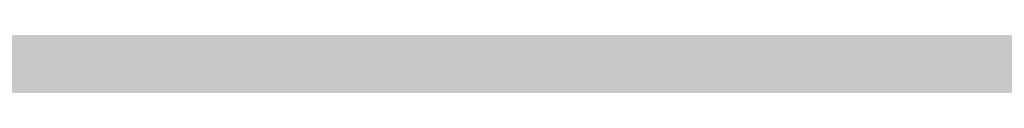
# Model space of a CAD drawing. Units: inches. Extents: x 2091 to 2899, y 967 to 2217.
# Tile 175 of 256: x 2203.151632 to 2203.161218, y 1152.24748 to 1152.2479. Entities that reach past the tile are written whole.
import ezdxf

# ---------------------------------------------------------------- set-up
doc = ezdxf.new("R2010")
doc.units = ezdxf.units.IN
doc.layers.add('A-WALL-PATT', color=141, linetype='Continuous', lineweight=13, true_color=0xadddf7)

msp = doc.modelspace()

# ---------------------------------------------------------------- hatches: boundary and pattern name
at = {"layer": 'A-WALL-PATT'}
h = msp.add_hatch(color=256, dxfattribs=at)
h.dxf.hatch_style = 1
h.paths.add_polyline_path([(2803.1436027, 2050.9190588), (2203.1436027, 2050.9190588), (2203.1436027, 1090.9190588), (2803.1436027, 1090.9190588)])
h.paths.add_polyline_path([(2635.7988501, 1147.5404649), (2674.5240524, 1147.5404649, 0.376086), (2678.5296653, 1152.8802017), (2678.5296653, 1159.5564734, 0.333335), (2674.524319, 1163.561846), (2674.524319, 1163.5618504), (2674.524319, 1192.9343904), (2635.8059707, 1192.9343904), (2597.0876225, 1192.9343904), (2597.0876225, 1163.561846, 0.333335), (2593.0822761, 1159.5564734), (2593.0822761, 1152.8802017, 0.376086), (2597.087889, 1147.5404649)], flags=0)
h.paths.add_polyline_path([(2436.0104329, 1278.2407784, 0.000483), (2435.9526433, 1278.215027, -0.001328), (2435.9356253, 1278.1116934, -0.001711), (2436.1164401, 1278.0407583, 0.002185)], flags=0)
h.paths.add_polyline_path([(2794.1436027, 1143.4190588), (2794.1436027, 1347.4190588), (2543.3701706, 1347.4190588), (2543.3701706, 1351.9190588), (2794.1436027, 1351.9190588), (2794.1436027, 1392.7135549), (2793.9473982, 1392.7135549), (2793.9473982, 1473.5368999), (2794.1436027, 1473.5368999), (2794.1436027, 1531.9190588), (2650.1436027, 1531.9190588), (2650.1436027, 1536.4190588), (2794.1436027, 1536.4190588), (2794.1436027, 1692.4190588), (2609.3756095, 1692.4190588), (2609.3756095, 1644.4190588), (2604.8756095, 1644.4190588), (2604.8756095, 1744.9190588), (2609.3756095, 1744.9190588), (2609.3756095, 1696.9190588), (2794.1436027, 1696.9190588), (2794.1436027, 1780.9190588), (2609.6436027, 1780.9190588), (2493.8756095, 1780.9190588), (2493.8756095, 1785.4190588), (2609.6436027, 1785.4190588), (2794.1436027, 1785.4190588), (2794.1436027, 1847.9388214), (2793.9512217, 1847.9388214), (2793.9512217, 1928.7621663), (2794.1436027, 1928.7621663), (2794.1436027, 1941.4190588), (2614.1436027, 1941.4190588), (2614.1436027, 1821.4190588), (2609.6436027, 1821.4190588), (2609.6436027, 1941.4190588), (2392.1436027, 1941.4190588), (2392.1436027, 1819.9190588), (2387.6436027, 1819.9190588), (2387.6436027, 1941.4190588), (2212.1436027, 1941.4190588), (2212.1436027, 1783.9190588), (2392.1436027, 1783.9190588), (2392.1436027, 1780.9190588), (2212.1436027, 1780.9190588), (2212.1436027, 1629.4190588), (2387.6436027, 1629.4190588), (2387.6436027, 1744.9190588), (2392.1436027, 1744.9190588), (2392.1436027, 1627.9190588), (2317.1436027, 1627.9190588), (2317.1436027, 1551.4190588), (2317.1436027, 1536.4190588), (2459.3835909, 1536.4190588), (2459.3835909, 1602.3964802), (2463.8835909, 1602.3964802), (2463.8835909, 1531.9190588), (2456.6436027, 1531.9190588), (2456.6436027, 1529.9190588), (2452.1436027, 1529.9190588), (2452.1436027, 1531.9190588), (2312.6436027, 1531.9190588), (2312.6436027, 1551.4190588), (2306.1436027, 1551.4190588), (2306.1436027, 1555.9190588), (2308.1436027, 1555.9190588), (2308.1436027, 1551.4190588), (2312.6436027, 1551.4190588), (2312.6436027, 1627.9190588), (2212.1436027, 1627.9190588), (2212.1436027, 1555.9190588), (2270.1436027, 1555.9190588), (2270.1436027, 1551.4190588), (2212.1436027, 1551.4190588), (2212.1436027, 1351.9190588), (2272.1436027, 1351.9190588), (2272.1436027, 1347.4190588), (2212.1436027, 1347.4190588), (2212.1436027, 1275.4190588), (2308.1436027, 1275.4190588), (2308.1436027, 1351.9190588), (2452.1436027, 1351.9190588), (2452.1436027, 1493.9190588), (2456.6436027, 1493.9190588), (2456.6436027, 1347.4190588), (2312.6436027, 1347.4190588), (2312.6436027, 1270.9190588), (2212.1436027, 1270.9190588), (2212.1436027, 1099.9190588), (2281.2375229, 1099.9190588), (2282.8710413, 1110.9138034), (2282.0083413, 1116.9966034), (2278.5577413, 1121.4204034), (2268.2056413, 1128.0562034), (2272.0876413, 1128.0562034), (2273.8129413, 1131.9270034), (2279.4203413, 1134.6919034), (2285.0278413, 1135.2449034), (2287.6158413, 1137.4568034), (2288.0471413, 1138.0098034), (2289.3411413, 1140.7747034), (2291.0665413, 1139.6687034), (2292.3605413, 1135.2449034), (2295.3798413, 1136.9038034), (2296.2425413, 1135.7979034), (2297.1052413, 1133.0330034), (2300.1246413, 1138.0098034), (2303.1439413, 1138.0098034), (2304.4379413, 1135.7979034), (2303.1439413, 1133.5860034), (2306.5946413, 1134.6919034), (2307.8887413, 1133.0330034), (2310.9080413, 1135.2449034), (2313.9274413, 1134.1389034), (2315.6268599, 1132.4271023), (2308.3200413, 1117.5496034), (2290.2038413, 1109.8079034), (2288.9098413, 1103.1721034), (2289.2723086, 1099.9190588), (2434.9182274, 1099.9190588), (2431.5932274, 1124.7880588), (2429.9302274, 1169.5530588), (2430.9271848, 1240.5196942), (2435.6589255, 1238.1861258), (2437.1352274, 1196.5540588), (2438.7982274, 1143.9730588), (2442.6782274, 1111.9980588), (2446.5582274, 1099.9190588), (2794.1436027, 1099.9190588), (2794.1436027, 1138.9190588), (2548.0324471, 1138.9190588), (2548.0324471, 1143.4190588), (2548.0324471, 1148.8190588), (2546.6684571, 1148.0315588), (2528.6856919, 1179.1786218, 0.256256), (2512.0324471, 1148.8190588), (2512.0324471, 1143.4190588), (2512.0324471, 1138.9190588), (2507.5324471, 1138.9190588), (2507.5324471, 1143.4190588), (2507.5324471, 1148.8190588, 0.256256), (2490.8792023, 1179.1786218), (2472.8964371, 1148.0315588), (2471.5324471, 1148.8190588), (2471.5324471, 1143.4190588), (2467.0324471, 1143.4190588), (2467.0324471, 1269.9457858, 0.039061), (2460.9099871, 1273.5800588), (2467.0324471, 1273.5800588), (2467.0324471, 1286.3253638, 0.014511), (2465.2161944, 1286.7619052), (2467.0324471, 1287.0525761), (2467.0324471, 1323.4190588), (2471.5324471, 1323.4190588), (2471.5324471, 1148.8190588), (2489.5324471, 1179.9959734), (2490.8964371, 1179.2084734), (2490.8792023, 1179.1786218, -0.256256), (2507.5324471, 1148.8190588), (2507.5324471, 1143.4190588), (2512.0324471, 1143.4190588), (2512.0324471, 1148.8190588, -0.256256), (2528.6856919, 1179.1786218), (2528.6684571, 1179.2084734), (2530.0324471, 1179.9959734), (2548.0324471, 1148.8190588), (2548.0324471, 1143.4190588)], flags=16)
h.paths.add_polyline_path([(2607.7685461, 1200.9450832), (2607.7685461, 1265.0306251), (2597.0876225, 1281.0520106), (2619.7845852, 1281.0520106), (2627.795278, 1337.1268598), (2635.7988501, 1337.1268598), (2643.8166634, 1337.1268598), (2651.8273562, 1281.0520106), (2674.524319, 1281.0520106), (2663.8433953, 1265.0306251), (2663.8433953, 1200.9450832), (2635.8059707, 1200.9450832)], flags=0)
edge = h.paths.add_edge_path(flags=0)
edge.add_ellipse((13303.8962153, 1272.9987247), major_axis=(-10595.3130399, 0.0000005), ratio=0.842303870086, start_angle=0.62823721906, end_angle=0.64655409989, ccw=False)
edge.add_ellipse((2711.7004495, 1156.8526781), major_axis=(2.2197691, 0), ratio=0.84230387, start_angle=111.5352435, end_angle=180.6282372, ccw=False)
edge.add_ellipse((13303.1562922, 1272.9987246), major_axis=(-10593.0263064, 0), ratio=0.842303869544, start_angle=0.52827147182, end_angle=0.64655409706, ccw=False)
edge.add_line((2710.7645961, 1175.3332951), (2710.1299858, 1175.3332951))
edge.add_ellipse((2710.1299858, 1176.5797752), major_axis=(1.4798461, 0), ratio=0.84230387, start_angle=180, end_angle=270, ccw=False)
edge.add_line((2708.6501397, 1176.5797752), (2708.6501397, 1200.7829144))
edge.add_ellipse((2710.1299858, 1200.7829144), major_axis=(1.4798461, 0), ratio=0.84230387, start_angle=90, end_angle=180, ccw=False)
edge.add_line((2710.1299858, 1202.0293944), (2710.4650752, 1202.0293944))
edge.add_ellipse((13303.1562922, 1272.9987246), major_axis=(-10593.0263064, 0), ratio=0.842303869544, start_angle=-0.09022908859, end_angle=0.38386677879, ccw=False)
edge.add_ellipse((2710.1299858, 1290.9270308), major_axis=(-1.4798461, 0), ratio=0.84230387, start_angle=0, end_angle=90, ccw=False)
edge.add_line((2708.6501397, 1290.9270308), (2708.6501397, 1315.13017))
edge.add_ellipse((2710.1299858, 1315.13017), major_axis=(-1.4798461, 0), ratio=0.84230387, start_angle=-90, end_angle=0, ccw=False)
edge.add_line((2710.1299858, 1316.3766501), (2710.7063141, 1316.3766501))
edge.add_ellipse((3238.4017202, 1296.2895655), major_axis=(528.2339998, 0), ratio=0.84230386954, start_angle=176.349572414, end_angle=177.820049686, ccw=False)
edge.add_ellipse((2775.0630432, 1071.4506962), major_axis=(313.3077613, 0), ratio=0.84230386954, start_angle=102.125965552, end_angle=103.780528989, ccw=False)
edge.add_ellipse((2775.0630432, 1078.3056979), major_axis=(-305.3028915, 0), ratio=0.84230386955, start_angle=-79.790461003, end_angle=-77.555372706, ccw=False)
edge.add_ellipse((2695.1417666, 1541.9753825), major_axis=(-250.9602162, 0), ratio=0.84230386954, start_angle=99.256566007, end_angle=102.554932644)
edge.add_line((2741.4103262, 1334.2142554), (2747.1325454, 1337.3784768))
edge.add_ellipse((2747.5386163, 1336.8574776), major_axis=(-0.739923, 0), ratio=0.84230387, start_angle=270, end_angle=307.9331305, ccw=False)
edge.add_ellipse((2747.5386163, 1336.8574776), major_axis=(-0.739923, 0), ratio=0.84230387, start_angle=232.0668695, end_angle=270, ccw=False)
edge.add_line((2747.9446872, 1337.3784768), (2753.6669064, 1334.2142554))
edge.add_ellipse((2799.935466, 1541.9753825), major_axis=(250.9602162, 0), ratio=0.84230386954, start_angle=257.445067356, end_angle=260.743433993)
edge.add_ellipse((2720.0141894, 1078.3056979), major_axis=(305.3028915, 0), ratio=0.84230386954, start_angle=77.555372707, end_angle=79.790461003, ccw=False)
edge.add_ellipse((2720.0141894, 1071.4506962), major_axis=(-313.3077613, 0), ratio=0.84230386954, start_angle=256.219471011, end_angle=257.874034448, ccw=False)
edge.add_ellipse((2256.6755124, 1296.2895655), major_axis=(-528.2339998, 0), ratio=0.84230386954, start_angle=182.179950314, end_angle=183.650427586, ccw=False)
edge.add_line((2784.3709184, 1316.3766501), (2784.9472468, 1316.3766501))
edge.add_ellipse((2784.9472468, 1315.13017), major_axis=(1.4798461, 0), ratio=0.84230387, start_angle=0, end_angle=90, ccw=False)
edge.add_line((2786.4270928, 1315.13017), (2786.4270928, 1290.9270308))
edge.add_ellipse((2784.9472468, 1290.9270308), major_axis=(1.4798461, 0), ratio=0.84230387, start_angle=270, end_angle=360, ccw=False)
edge.add_ellipse((-7808.0790596, 1272.9987246), major_axis=(10593.0263063, 0), ratio=0.842303869544, start_angle=-0.38386677879, end_angle=0.09022908859, ccw=False)
edge.add_line((2784.6121574, 1202.0293944), (2784.9472468, 1202.0293944))
edge.add_ellipse((2784.9472468, 1200.7829144), major_axis=(1.4798461, 0), ratio=0.84230387, start_angle=0, end_angle=90, ccw=False)
edge.add_line((2786.4270928, 1200.7829144), (2786.4270928, 1176.5797752))
edge.add_ellipse((2784.9472468, 1176.5797752), major_axis=(-1.4798461, 0), ratio=0.84230387, start_angle=90, end_angle=180, ccw=False)
edge.add_line((2784.9472468, 1175.3332951), (2784.3126365, 1175.3332951))
edge.add_ellipse((-7808.0790596, 1272.9987246), major_axis=(10593.0263063, 0), ratio=0.842303869544, start_angle=-0.61864319632, end_angle=-0.52827147182, ccw=False)
edge.add_ellipse((2783.3767831, 1156.8526781), major_axis=(-2.2197691, 0), ratio=0.84230387, start_angle=179.3717628, end_angle=248.4647566, ccw=False)
edge.add_ellipse((-7808.8189826, 1272.9987246), major_axis=(-10595.3130398, 0.0000036), ratio=0.842303865762, start_angle=179.3534459226, end_angle=179.37176280343, ccw=False)
edge.add_ellipse((2780.2973026, 1153.500793), major_axis=(-5.2464256, 0), ratio=0.84230387, start_angle=90, end_angle=179.3534459, ccw=False)
edge.add_line((2780.2973026, 1149.0817084), (2714.77993, 1149.0817084))
edge.add_ellipse((2714.77993, 1153.500793), major_axis=(5.2464256, 0), ratio=0.84230387, start_angle=180.6465541, end_angle=270, ccw=False)
edge = h.paths.add_edge_path(flags=0)
edge.add_line((2718.1873674, 1151.0078329), (2718.1873674, 1170.4723638))
edge.add_ellipse((2721.1470595, 1170.4723638), major_axis=(-2.9596921, 0), ratio=0.84230387, start_angle=-90, end_angle=0, ccw=False)
edge.add_line((2721.1470595, 1172.965324), (2773.9301731, 1172.965324))
edge.add_ellipse((2773.9301731, 1170.4723638), major_axis=(-2.9596921, 0), ratio=0.84230387, start_angle=180, end_angle=270, ccw=False)
edge.add_line((2776.8898652, 1170.4723638), (2776.8898652, 1151.0078329))
edge.add_line((2776.8898652, 1151.0078329), (2718.1873674, 1151.0078329))
edge = h.paths.add_edge_path(flags=0)
edge.add_line((2718.1873674, 1180.2341502), (2718.1873674, 1199.0578342))
edge.add_ellipse((2747.5386163, 1320.3986402), major_axis=(147.0179239, 0), ratio=0.84230386954, start_angle=256.40186531, end_angle=283.59813469)
edge.add_line((2776.8898652, 1199.0578342), (2776.8898652, 1180.2341502))
edge.add_ellipse((2747.5386163, 1301.5749562), major_axis=(147.0179239, 0), ratio=0.84230386954, start_angle=256.40186531, end_angle=283.59813469, ccw=False)
edge = h.paths.add_edge_path(flags=0)
edge.add_ellipse((13303.1562922, 1272.9987246), major_axis=(-10591.5464603, 0), ratio=0.842303869555, start_angle=0.05559431352, end_angle=0.37776419393, ccw=False)
edge.add_line((2711.6168595, 1262.7217103), (2715.6674076, 1249.4953957))
edge.add_ellipse((6413.8919626, 1241.691919), major_axis=(-3698.2361592, 0), ratio=0.842303869547, start_angle=-0.120897369, end_angle=0.3640763489)
edge.add_line((2715.7610383, 1218.1924547), (2711.9343065, 1203.167361))
edge = h.paths.add_edge_path(flags=0)
edge.add_line((2718.1873674, 1251.074566), (2716.0024854, 1267.4504351))
edge.add_ellipse((2742.1511746, 1202.1895399), major_axis=(81.7725845, 0), ratio=0.8423038695, start_angle=94.277420963, end_angle=111.834953797, ccw=False)
edge.add_line((2737.0097482, 1270.9306255), (2758.0674844, 1270.9306255))
edge.add_ellipse((2752.926058, 1202.1895399), major_axis=(81.7725845, 0), ratio=0.8423038695, start_angle=68.165046203, end_angle=85.722579037, ccw=False)
edge.add_line((2779.0747472, 1267.4504351), (2776.8898652, 1251.074566))
edge.add_ellipse((2750.3380588, 1187.8853558), major_axis=(79.5796641, 0), ratio=0.8423038695, start_angle=67.208085122, end_angle=85.129930403)
edge.add_line((2756.0346562, 1254.7436557), (2739.0425764, 1254.7436557))
edge.add_ellipse((2744.7391738, 1187.8853558), major_axis=(79.5796641, 0), ratio=0.8423038695, start_angle=94.870069597, end_angle=112.791914878)
edge = h.paths.add_edge_path(flags=0)
edge.add_line((2783.1429261, 1203.167361), (2779.3161943, 1218.1924547))
edge.add_ellipse((-918.81473, 1241.691919), major_axis=(3698.2361592, 0), ratio=0.842303869546, start_angle=-0.3640763489, end_angle=0.120897369)
edge.add_line((2779.409825, 1249.4953957), (2783.4603731, 1262.7217103))
edge.add_ellipse((-7808.0790596, 1272.9987246), major_axis=(-10591.5464603, 0), ratio=0.84230386954, start_angle=179.6222358061, end_angle=179.94440568651, ccw=False)
edge = h.paths.add_edge_path(flags=0)
edge.add_ellipse((2734.2008921, 1286.6904402), major_axis=(-0.3566086, 6.3400775), ratio=0.603833576, start_angle=89.00201428, end_angle=253.65740805, ccw=False)
edge.add_line((2730.3690013, 1286.5418057), (2730.3690013, 1301.3519803))
edge.add_line((2730.3690013, 1301.3519803), (2735.9133107, 1305.2148028))
edge.add_ellipse((2736.3849168, 1304.7345612), major_axis=(0.739923, 0), ratio=0.84230387, start_angle=90, end_angle=134.4802109, ccw=False)
edge.add_line((2736.3849168, 1305.3578013), (2738.0327829, 1305.3578013))
edge.add_line((2738.0327829, 1305.3578013), (2738.0327829, 1307.7079274))
edge.add_ellipse((2794.201642, 1307.7079274), major_axis=(56.168859, 0), ratio=0.8423038695, start_angle=150.5614304, end_angle=180, ccw=False)
edge.add_ellipse((2700.8755906, 1307.7079274), major_axis=(-56.168859, 0), ratio=0.8423038695, start_angle=180, end_angle=209.4385696, ccw=False)
edge.add_line((2757.0444497, 1307.7079274), (2757.0444497, 1305.3578013))
edge.add_line((2757.0444497, 1305.3578013), (2758.6923157, 1305.3578013))
edge.add_ellipse((2758.6923157, 1304.7345612), major_axis=(-0.739923, 0), ratio=0.84230387, start_angle=225.5197891, end_angle=270, ccw=False)
edge.add_line((2759.1639219, 1305.2148028), (2764.7082312, 1301.3519803))
edge.add_line((2764.7082312, 1301.3519803), (2764.7082312, 1286.5418057))
edge.add_ellipse((2760.8763405, 1286.6904402), major_axis=(0.3566086, 6.3400775), ratio=0.603833576, start_angle=106.34259195, end_angle=270.99798572, ccw=False)
edge.add_line((2757.0444497, 1285.7970896), (2757.0444497, 1307.7079274))
edge.add_ellipse((2700.8755906, 1307.7079274), major_axis=(-56.168859, 0), ratio=0.8423038695, start_angle=180, end_angle=209.4385696)
edge.add_ellipse((2794.201642, 1307.7079274), major_axis=(56.168859, 0), ratio=0.8423038695, start_angle=150.5614304, end_angle=180)
edge.add_line((2738.0327829, 1307.7079274), (2738.0327829, 1285.7970896))
h.paths.add_polyline_path([(2417.8122727, 1104.449704), (2413.4922727, 1102.529704), (2410.6122727, 1103.969704), (2409.1722727, 1106.369704), (2407.2522727, 1107.329704), (2406.2922727, 1109.729704), (2405.3322727, 1114.049704), (2405.3322727, 1117.889704), (2406.2922727, 1120.129704), (2407.2522727, 1119.809704), (2408.8483218, 1118.3276585), (2410.1739451, 1119.4241703), (2410.2112727, 1120.405704), (2411.0407305, 1121.4190541), (2410.6992727, 1119.858704), (2410.1739451, 1119.4241703), (2410.0884515, 1117.1761095), (2411.1328361, 1116.2063237), (2413.9722727, 1119.329704), (2416.8522727, 1120.769704), (2416.8697209, 1120.7987842), (2417.0350713, 1119.4051162), (2417.8962134, 1118.1433844), (2418.2922727, 1118.369704), (2419.5444467, 1120.0392692), (2419.3609153, 1118.387487), (2419.0321078, 1119.3561507), (2418.3989394, 1118.5119262), (2419.2522727, 1114.529704), (2418.7940909, 1107.1987949)], flags=0)
h.paths.add_polyline_path([(2508.8701706, 1347.4190588), (2508.3701706, 1347.4190588), (2508.3701706, 1351.9190588), (2508.8701706, 1351.9190588)], flags=0)
h.paths.add_polyline_path([(2473.3701706, 1347.4190588), (2472.3701706, 1347.4190588), (2467.8701706, 1347.4190588), (2467.8701706, 1455.4190588), (2472.3701706, 1455.4190588), (2472.3701706, 1352.4190588), (2473.3701706, 1352.4190588)], flags=0)
h.paths.add_polyline_path([(2352.106244, 1217.4461971), (2349.226244, 1218.8861971), (2347.786244, 1221.2861971), (2345.866244, 1222.2461971), (2344.906244, 1224.6461971), (2343.946244, 1228.9661971), (2343.946244, 1232.8061971), (2344.906244, 1235.0461971), (2345.866244, 1234.7261971), (2347.4622931, 1233.2441515), (2348.7879164, 1234.3406634), (2348.825244, 1235.3221971), (2349.6547018, 1236.3355471), (2349.313244, 1234.7751971), (2348.7879164, 1234.3406634), (2348.7024228, 1232.0926025), (2349.7468074, 1231.1228168), (2352.586244, 1234.2461971), (2355.466244, 1235.6861971), (2355.4836921, 1235.7152773), (2355.6490426, 1234.3216093), (2356.5101846, 1233.0598774), (2356.906244, 1233.2861971), (2358.1584179, 1234.9557623), (2357.9748866, 1233.3039801), (2357.6460791, 1234.2726438), (2357.0129107, 1233.4284193), (2357.866244, 1229.4461971), (2357.4080622, 1222.115288), (2356.426244, 1219.3661971)], flags=0)
h.paths.add_polyline_path([(2348.2967999, 1112.2244204), (2347.0137999, 1112.3104204), (2345.5297999, 1114.1274204), (2345.7317999, 1115.8584204), (2346.8117999, 1116.9824204), (2346.8117999, 1114.6464204), (2345.8667999, 1114.2144204), (2346.8797999, 1114.3004204)], flags=0)
h.paths.add_polyline_path([(2347.0137999, 1110.9264204), (2346.2717999, 1110.4934204), (2346.6097999, 1111.1864204)], flags=0)
h.paths.add_polyline_path([(2345.8667999, 1118.1944204), (2345.5297999, 1117.3294204), (2343.7077999, 1118.0214204), (2344.3827999, 1118.6264204)], flags=0)
h.paths.add_polyline_path([(2346.6767999, 1109.2824204), (2346.0697999, 1108.0714204), (2345.8667999, 1110.0614204)], flags=0)
h.paths.add_polyline_path([(2345.0567999, 1119.7514204), (2343.6397999, 1119.7514204), (2343.9777999, 1121.1354204)], flags=0)
h.paths.add_polyline_path([(2345.2597999, 1116.5504204), (2345.1247999, 1115.8584204), (2344.9217999, 1115.6854204), (2344.7197999, 1116.3774204)], flags=0)
h.paths.add_polyline_path([(2345.6647999, 1112.3104204), (2345.4617999, 1111.5324204), (2344.0447999, 1111.9644204), (2344.6517999, 1112.5704204)], flags=0)
h.paths.add_polyline_path([(2345.1917999, 1113.3494204), (2344.4497999, 1113.8684204), (2344.7197999, 1114.3874204)], flags=0)
h.paths.add_polyline_path([(2344.6517999, 1116.8094204), (2344.1797999, 1115.6854204), (2344.6517999, 1115.3394204), (2343.9097999, 1114.9064204), (2343.0327999, 1115.9444204), (2343.6397999, 1116.4634204)], flags=0)
h.paths.add_polyline_path([(2345.8667999, 1106.6864204), (2344.9897999, 1105.5624204), (2344.5167999, 1106.6004204)], flags=0)
h.paths.add_polyline_path([(2344.8547999, 1110.0614204), (2344.5167999, 1109.2824204), (2344.1127999, 1109.7154204)], flags=0)
h.paths.add_polyline_path([(2344.0447999, 1113.5224204), (2343.4377999, 1113.0894204), (2342.7627999, 1113.9544204)], flags=0)
h.paths.add_polyline_path([(2344.3147999, 1111.0124204), (2342.9647999, 1110.3204204), (2342.9647999, 1111.0994204)], flags=0)
h.paths.add_polyline_path([(2345.1247999, 1104.6974204), (2344.5847999, 1103.7454204), (2344.4497999, 1104.2644204)], flags=0)
h.paths.add_polyline_path([(2342.8297999, 1121.2224204), (2341.7497999, 1120.5304204), (2340.5357999, 1121.0494204), (2340.1307999, 1121.8284204), (2340.6707999, 1122.9524204), (2341.1427999, 1121.8284204), (2341.6147999, 1122.0014204)], flags=0)
h.paths.add_polyline_path([(2342.9647999, 1119.7514204), (2343.0327999, 1118.4534204), (2342.0877999, 1118.0214204), (2342.0197999, 1119.4914204)], flags=0)
h.paths.add_polyline_path([(2342.6947999, 1116.8964204), (2341.9527999, 1116.6364204), (2342.0197999, 1117.3294204)], flags=0)
h.paths.add_polyline_path([(2343.0327999, 1112.2244204), (2342.0197999, 1111.7914204), (2341.5477999, 1112.2244204), (2342.3577999, 1113.3494204)], flags=0)
h.paths.add_polyline_path([(2343.7747999, 1104.4374204), (2342.6277999, 1102.8804204), (2342.6947999, 1104.6104204), (2343.4377999, 1105.1294204)], flags=0)
h.paths.add_polyline_path([(2342.0197999, 1115.0794204), (2340.8057999, 1115.5124204), (2340.9407999, 1116.3774204)], flags=0)
h.paths.add_polyline_path([(2341.4807999, 1120.0974204), (2341.4807999, 1119.4054204), (2341.0757999, 1119.5784204), (2341.1427999, 1120.0974204)], flags=0)
h.paths.add_polyline_path([(2341.8177999, 1114.4734204), (2340.9407999, 1113.0894204), (2340.8057999, 1114.5604204)], flags=0)
h.paths.add_polyline_path([(2341.1427999, 1118.5404204), (2340.9407999, 1116.9824204), (2339.0507999, 1117.6754204), (2339.0507999, 1118.6264204)], flags=0)
h.paths.add_polyline_path([(2342.6947999, 1101.6684204), (2341.9527999, 1101.8414204), (2342.5597999, 1102.3614204)], flags=0)
h.paths.add_polyline_path([(2340.3327999, 1119.6654204), (2338.4437999, 1119.5784204), (2337.9037999, 1120.3574204), (2339.6577999, 1120.6164204)], flags=0)
h.paths.add_polyline_path([(2340.3327999, 1115.3394204), (2340.0627999, 1113.6954204), (2339.3877999, 1115.3394204)], flags=0)
h.paths.add_polyline_path([(2341.8177999, 1103.8314204), (2341.5477999, 1102.8804204), (2341.1427999, 1103.6584204)], flags=0)
h.paths.add_polyline_path([(2339.0507999, 1122.8664204), (2337.2957999, 1121.8284204), (2337.0937999, 1123.1254204), (2337.7687999, 1123.8184204)], flags=0)
h.paths.add_polyline_path([(2339.1177999, 1121.7414204), (2338.8477999, 1121.2224204), (2338.1737999, 1121.0494204), (2338.3757999, 1121.5684204)], flags=0)
h.paths.add_polyline_path([(2339.1857999, 1119.3194204), (2338.6457999, 1118.7134204), (2338.2407999, 1118.1074204), (2338.2407999, 1118.8864204)], flags=0)
h.paths.add_polyline_path([(2341.1427999, 1101.9284204), (2340.6027999, 1101.2364204), (2340.0627999, 1101.8414204), (2340.6027999, 1102.3614204)], flags=0)
h.paths.add_polyline_path([(2337.6337999, 1117.7614204), (2336.6207999, 1118.2804204), (2337.2957999, 1118.9724204)], flags=0)
h.paths.add_polyline_path([(2336.8237999, 1119.5784204), (2334.7987999, 1118.9724204), (2335.2037999, 1120.3574204), (2336.5537999, 1120.8764204)], flags=0)
h.paths.add_polyline_path([(2339.1177999, 1100.4574204), (2337.3637999, 1100.5434204), (2336.7557999, 1101.2364204)], flags=0)
h.paths.add_polyline_path([(2336.3507999, 1122.4334204), (2336.0137999, 1121.9144204), (2334.9337999, 1122.4334204), (2334.5287999, 1123.4714204), (2335.7437999, 1122.7794204)], flags=0)
h.paths.add_polyline_path([(2334.7317999, 1120.8764204), (2334.2587999, 1120.3574204), (2334.0567999, 1120.7894204), (2334.5967999, 1121.3084204)], flags=0)
h.paths.add_polyline_path([(2334.4617999, 1122.1744204), (2332.5717999, 1121.3084204), (2331.3567999, 1122.1744204), (2332.0997999, 1122.8664204)], flags=0)
h.paths.add_polyline_path([(2334.2587999, 1118.5404204), (2333.3817999, 1118.4534204), (2333.6517999, 1119.3194204)], flags=0)
h.paths.add_polyline_path([(2335.5417999, 1102.2744204), (2334.1917999, 1102.6204204), (2335.2717999, 1103.3124204)], flags=0)
h.paths.add_polyline_path([(2332.7067999, 1119.6654204), (2331.6947999, 1120.4434204), (2332.5047999, 1120.7894204)], flags=0)
h.paths.add_polyline_path([(2334.7317999, 1101.1494204), (2333.5167999, 1101.5824204), (2333.9887999, 1101.7554204)], flags=0)
h.paths.add_polyline_path([(2332.6397999, 1116.6364204), (2331.0867999, 1116.2904204), (2331.9647999, 1118.1944204)], flags=0)
h.paths.add_polyline_path([(2330.7497999, 1121.5684204), (2330.2767999, 1120.2704204), (2328.5227999, 1119.3194204), (2328.9947999, 1121.0494204)], flags=0)
h.paths.add_polyline_path([(2330.7497999, 1118.6264204), (2330.0077999, 1117.5024204), (2329.8727999, 1118.0214204)], flags=0)
h.paths.add_polyline_path([(2332.0997999, 1102.3614204), (2330.5467999, 1102.0144204), (2331.6947999, 1102.9664204)], flags=0)
h.paths.add_polyline_path([(2329.5347999, 1113.6084204), (2329.0627999, 1112.3104204), (2328.5897999, 1113.3494204)], flags=0)
h.paths.add_polyline_path([(2328.3877999, 1117.8484204), (2327.5097999, 1116.5504204), (2327.1727999, 1117.7614204)], flags=0)
h.paths.add_polyline_path([(2329.7377999, 1106.5134204), (2329.5347999, 1105.3024204), (2328.2527999, 1106.0814204)], flags=0)
h.paths.add_polyline_path([(2328.6577999, 1114.3874204), (2328.0497999, 1114.1274204), (2328.3197999, 1114.9064204)], flags=0)
h.paths.add_polyline_path([(2328.3197999, 1112.2244204), (2327.1057999, 1112.1374204), (2326.7007999, 1112.6564204)], flags=0)
h.paths.add_polyline_path([(2326.9027999, 1115.2524204), (2326.7007999, 1114.1274204), (2325.2157999, 1113.6084204), (2326.0927999, 1115.3394204)], flags=0)
h.paths.add_polyline_path([(2326.6327999, 1108.3304204), (2326.0927999, 1107.3794204), (2325.8907999, 1108.5034204), (2326.4977999, 1109.1094204)], flags=0)
h.paths.add_polyline_path([(2615.1436027, 1531.9190588), (2609.6436027, 1531.9190588), (2609.6436027, 1620.4190588), (2614.1436027, 1620.4190588), (2614.1436027, 1536.4190588), (2615.1436027, 1536.4190588)], flags=0)
h.paths.add_polyline_path([(2545.1436027, 1563.4190588), (2464.1436027, 1563.4190588), (2464.1436027, 1632.4190588), (2509.1436027, 1632.4190588), (2509.1436027, 1627.9190588), (2509.1436027, 1603.9190588), (2468.6436027, 1603.9190588), (2468.6436027, 1567.9190588), (2540.6436027, 1567.9190588), (2540.6436027, 1591.9190588), (2545.1436027, 1591.9190588)], flags=0)
h.paths.add_polyline_path([(2388.9690483, 1549.985735), (2357.4341811, 1549.985735), (2357.4341811, 1623.3607783), (2399.3627772, 1623.3607783), (2435.6894654, 1623.3607783), (2435.5925469, 1602.5592734), (2435.5925469, 1602.3964802), (2388.9690483, 1602.3964802)], flags=0)
h.paths.add_polyline_path([(2388.8806282, 1555.8091511), (2374.9044295, 1555.8091511), (2374.9044295, 1600.5715641), (2374.9044295, 1615.4576454), (2406.3508766, 1615.4576454), (2406.3508766, 1618.9394309), (2412.1742927, 1615.4576454), (2406.3508766, 1611.9758599), (2406.3508766, 1615.4576454), (2388.8806282, 1615.4576454)], flags=0)
h.paths.add_polyline_path([(2568.8756095, 1644.4190588), (2453.3756095, 1644.4190588), (2453.3756095, 1785.4190588), (2457.8756095, 1785.4190588), (2457.8756095, 1648.9190588), (2568.8756095, 1648.9190588)], flags=0)
h.paths.add_polyline_path([(2212.1436027, 1945.9190588), (2212.1436027, 2041.9190588), (2794.1436027, 2041.9190588), (2794.1436027, 1945.9190588)], flags=16)
h.paths.add_polyline_path([(2271.0827276, 1964.3172377), (2776.852968, 1964.3172377), (2776.852968, 2037.1696226), (2271.0827276, 2037.1696226)], flags=8)
h.paths.add_polyline_path([(2380.6492852, 1536.8241435), (2461.0408087, 1536.8241435), (2461.0408087, 1554.6525871), (2380.6492852, 1554.6525871)], flags=8)
h.paths.add_polyline_path([(2240.7557092, 1609.7254508), (2309.1858294, 1609.7254508), (2309.1858294, 1617.6982037), (2240.7557092, 1617.6982037)], flags=8)
h.paths.add_polyline_path([(2212.6772554, 1313.5041021), (2282.5915203, 1313.5041021), (2282.5915203, 1322.7452389), (2212.6772554, 1322.7452389)], flags=8)
h.paths.add_polyline_path([(2457.111976, 1114.778574), (2558.4815807, 1114.778574), (2558.4815807, 1142.2196823), (2457.111976, 1142.2196823)], flags=8)
h.paths.add_polyline_path([(2473.4423372, 1273.0100672), (2604.6412257, 1273.0100672), (2604.6412257, 1318.3469349), (2473.4423372, 1318.3469349)], flags=8)
h.paths.add_polyline_path([(2638.8763024, 1626.9774316), (2684.2503675, 1627.9767377), (2684.0384825, 1637.5974944), (2638.6644174, 1636.5981884)], flags=8)
h.paths.add_polyline_path([(2537.5905538, 1453.7934466), (2628.3895472, 1453.7934466), (2628.3895472, 1475.3448114), (2537.5905538, 1475.3448114)], flags=8)
h.paths.add_polyline_path([(2504.1376376, 1714.6323972), (2554.6471875, 1714.6323972), (2554.6471875, 1730.2377115), (2504.1376376, 1730.2377115)], flags=8)
h.paths.add_polyline_path([(2487.5011806, 1575.6518716), (2535.0971214, 1575.6518716), (2535.0971214, 1598.3776456), (2487.5011806, 1598.3776456)], flags=8)
h.paths.add_polyline_path([(2709.0994004, 1735.7102784), (2740.0166009, 1735.7102784), (2740.0166009, 1749.9376406), (2709.0994004, 1749.9376406)], flags=8)
h.paths.add_polyline_path([(2442.4384239, 1792.1716575), (2564.7288353, 1792.1716575), (2564.7288353, 1842.0001626), (2442.4384239, 1842.0001626)], flags=8)
h.paths.add_polyline_path([(2655.8158012, 1809.6440763), (2789.5201425, 1806.6937963), (2790.0849768, 1832.2916379), (2656.3806355, 1835.2419179)], flags=8)
h.paths.add_polyline_path([(2234.8426972, 1797.7201432), (2368.5928512, 1794.7688523), (2369.1607182, 1820.504132), (2235.4105642, 1823.4554229)], flags=8)
h.paths.add_polyline_path([(2245.1384659, 1644.0063348), (2398.4277329, 1640.6238997), (2398.9948417, 1666.3248199), (2245.7055747, 1669.7072549)], flags=8)
h.paths.add_polyline_path([(2306.1428474, 1431.1685186), (2413.7683138, 1428.7936873), (2414.3331481, 1454.3915289), (2306.7076817, 1456.7663602)], flags=8)
h.paths.add_polyline_path([(2306.834582, 1458.2331447), (2393.3804836, 1456.3234487), (2393.9328082, 1481.3543583), (2307.3869066, 1483.2640542)], flags=8)

doc.saveas('drawing.dxf')
